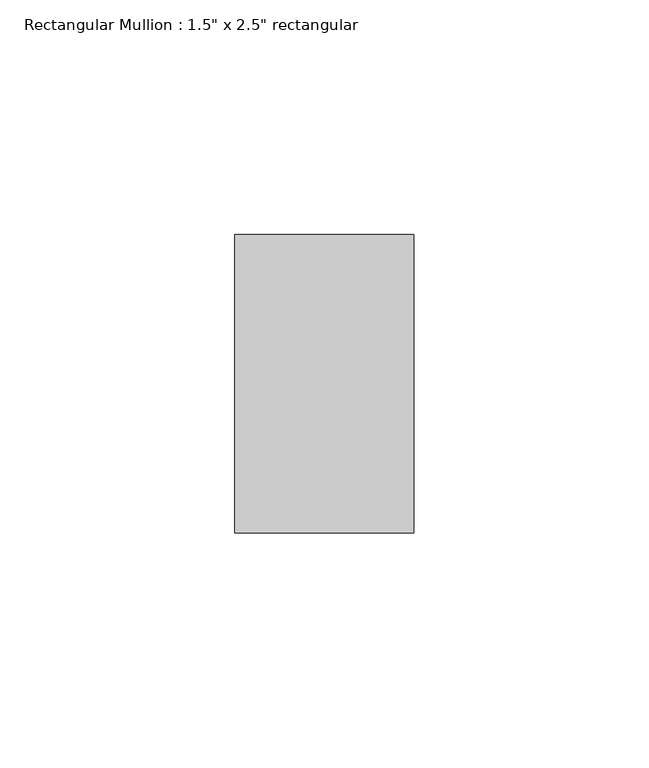
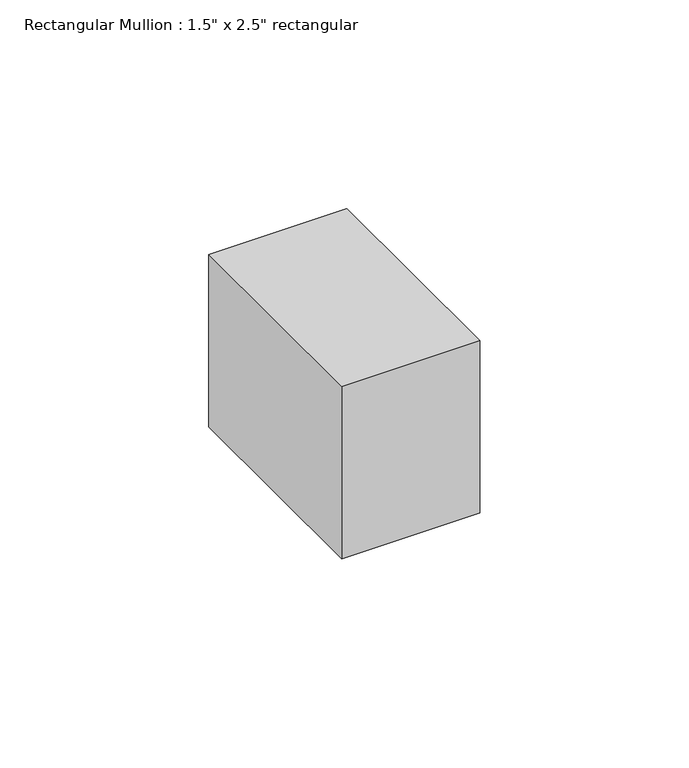
"""IFC4 building model written with IfcOpenShell, lengths in millimetres: member geometry."""

from ifc_helpers import new_model, si_unit, frame, origin, place, context, project, spatial, polyline, outline, extrude, source, transform, mapped, element, save


def member_6356c2c7(model_context):
    return source(origin(), model_context, "Body", "SweptSolid", [
        extrude(outline(polyline([(19.05, 31.75), (19.05, -31.75), (-19.05, -31.75), (-19.05, 31.75), (19.05, 31.75)])), frame((0.0, 0.0, -50.3801359), z_axis=(0.0, 0.0, 1.0), x_axis=(1.0, 0.0, 0.0)), (0.0, 0.0, 1.0), 50.3801359),
    ])


if __name__ == "__main__":
    model = new_model("IFC4")
    model_context = context("Model", 3, world=origin())
    ifc_project = project(units=[si_unit("LENGTHUNIT", "METRE", prefix="MILLI")], contexts=[model_context])
    site = spatial("IfcSite", under=ifc_project)
    building = spatial("IfcBuilding", under=site)
    placement = place(None, origin())
    member_shape = member_6356c2c7(model_context)
    element("IfcMember", 1, ObjectType="Rectangular Mullion : 1.5\" x 2.5\" rectangular", at=placement, inside=building, context=model_context, shape_type="MappedRepresentation", body=[
        mapped(member_shape, transform((0.0, 0.0, 0.0), x_axis=(1.0, 0.0, 0.0), y_axis=(0.0, 1.0, 0.0), z_axis=(0.0, 0.0, 1.0))),
    ])
    save(model, "model.ifc")

# Revit data of these elements
# Type "Rectangular Mullion : 1.5\" x 2.5\" rectangular"
#   built-in parameter 1007304 = 0.208333 (stored number, unit not read)
#   built-in parameter 1007301 = 0.0625 (stored number, unit not read)
#   built-in parameter 1007300 = 0.0625 (stored number, unit not read)
